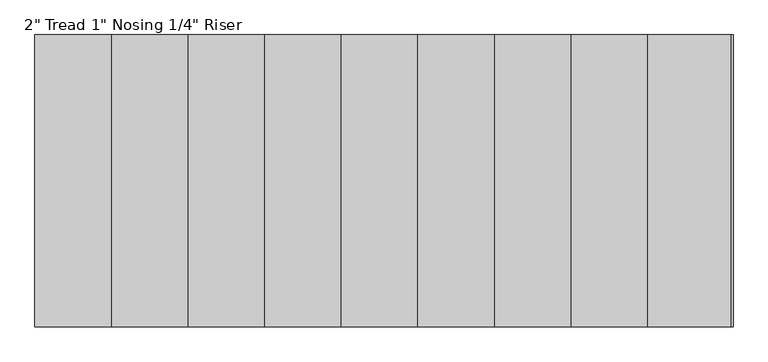
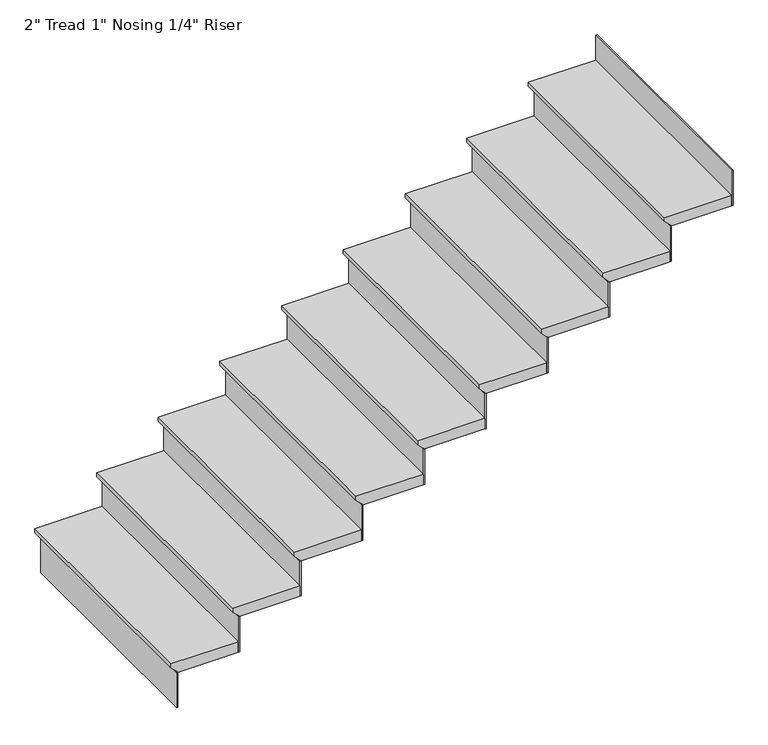
"""IFC4 building model written with IfcOpenShell, lengths in millimetres: stair flight geometry."""

from ifc_helpers import new_model, si_unit, frame, origin, place, context, project, spatial, polyline, outline, extrude, source, transform, mapped, element, save


def stair_flight_e984555f(model_context):
    return source(origin(), model_context, "Body", "SweptSolid", [
        extrude(outline(polyline([(1524.0, -13071.6750862), (1524.0, -13376.4750862), (1504.95, -13376.4750862), (1479.55, -13351.0750862), (1473.2, -13351.0750862), (1473.2, -13071.6750862), (1524.0, -13071.6750862)])), frame((0.0, 7319.8620171, 0.0), z_axis=(0.0, 1.0, 0.0), x_axis=(0.0, 0.0, 1.0)), (0.0, 0.0, 1.0), 1066.8),
        extrude(outline(polyline([(-13344.7250862, 7319.8620171), (-13351.0750862, 7319.8620171), (-13351.0750862, 8386.6620171), (-13344.7250862, 8386.6620171), (-13344.7250862, 7319.8620171)])), frame((0.0, 0.0, 1303.8666667), z_axis=(0.0, 0.0, 1.0), x_axis=(1.0, 0.0, 0.0)), (0.0, 0.0, 1.0), 169.3333333),
        extrude(outline(polyline([(-10830.1250862, 7319.8620171), (-10836.4750862, 7319.8620171), (-10836.4750862, 8386.6620171), (-10830.1250862, 8386.6620171), (-10830.1250862, 7319.8620171)])), frame((0.0, 0.0, 2827.8666667), z_axis=(0.0, 0.0, 1.0), x_axis=(1.0, 0.0, 0.0)), (0.0, 0.0, 1.0), 169.3333333),
        extrude(outline(polyline([(-13065.3250862, 7319.8620171), (-13071.6750862, 7319.8620171), (-13071.6750862, 8386.6620171), (-13065.3250862, 8386.6620171), (-13065.3250862, 7319.8620171)])), frame((0.0, 0.0, 1473.2), z_axis=(0.0, 0.0, 1.0), x_axis=(1.0, 0.0, 0.0)), (0.0, 0.0, 1.0), 169.3333333),
        extrude(outline(polyline([(1693.3333333, -12792.2750862), (1693.3333333, -13097.0750862), (1674.2833333, -13097.0750862), (1648.8833333, -13071.6750862), (1642.5333333, -13071.6750862), (1642.5333333, -12792.2750862), (1693.3333333, -12792.2750862)])), frame((0.0, 7319.8620171, 0.0), z_axis=(0.0, 1.0, 0.0), x_axis=(0.0, 0.0, 1.0)), (0.0, 0.0, 1.0), 1066.8),
        extrude(outline(polyline([(-12785.9250862, 7319.8620171), (-12792.2750862, 7319.8620171), (-12792.2750862, 8386.6620171), (-12785.9250862, 8386.6620171), (-12785.9250862, 7319.8620171)])), frame((0.0, 0.0, 1642.5333333), z_axis=(0.0, 0.0, 1.0), x_axis=(1.0, 0.0, 0.0)), (0.0, 0.0, 1.0), 169.3333333),
        extrude(outline(polyline([(1862.6666667, -12512.8750862), (1862.6666667, -12817.6750862), (1843.6166667, -12817.6750862), (1818.2166667, -12792.2750862), (1811.8666667, -12792.2750862), (1811.8666667, -12512.8750862), (1862.6666667, -12512.8750862)])), frame((0.0, 7319.8620171, 0.0), z_axis=(0.0, 1.0, 0.0), x_axis=(0.0, 0.0, 1.0)), (0.0, 0.0, 1.0), 1066.8),
        extrude(outline(polyline([(-12506.5250862, 7319.8620171), (-12512.8750862, 7319.8620171), (-12512.8750862, 8386.6620171), (-12506.5250862, 8386.6620171), (-12506.5250862, 7319.8620171)])), frame((0.0, 0.0, 1811.8666667), z_axis=(0.0, 0.0, 1.0), x_axis=(1.0, 0.0, 0.0)), (0.0, 0.0, 1.0), 169.3333333),
        extrude(outline(polyline([(2032.0, -12233.4750862), (2032.0, -12538.2750862), (2012.95, -12538.2750862), (1987.55, -12512.8750862), (1981.2, -12512.8750862), (1981.2, -12233.4750862), (2032.0, -12233.4750862)])), frame((0.0, 7319.8620171, 0.0), z_axis=(0.0, 1.0, 0.0), x_axis=(0.0, 0.0, 1.0)), (0.0, 0.0, 1.0), 1066.8),
        extrude(outline(polyline([(-12227.1250862, 7319.8620171), (-12233.4750862, 7319.8620171), (-12233.4750862, 8386.6620171), (-12227.1250862, 8386.6620171), (-12227.1250862, 7319.8620171)])), frame((0.0, 0.0, 1981.2), z_axis=(0.0, 0.0, 1.0), x_axis=(1.0, 0.0, 0.0)), (0.0, 0.0, 1.0), 169.3333333),
        extrude(outline(polyline([(2201.3333333, -11954.0750862), (2201.3333333, -12258.8750862), (2182.2833333, -12258.8750862), (2156.8833333, -12233.4750862), (2150.5333333, -12233.4750862), (2150.5333333, -11954.0750862), (2201.3333333, -11954.0750862)])), frame((0.0, 7319.8620171, 0.0), z_axis=(0.0, 1.0, 0.0), x_axis=(0.0, 0.0, 1.0)), (0.0, 0.0, 1.0), 1066.8),
        extrude(outline(polyline([(-11947.7250862, 7319.8620171), (-11954.0750862, 7319.8620171), (-11954.0750862, 8386.6620171), (-11947.7250862, 8386.6620171), (-11947.7250862, 7319.8620171)])), frame((0.0, 0.0, 2150.5333333), z_axis=(0.0, 0.0, 1.0), x_axis=(1.0, 0.0, 0.0)), (0.0, 0.0, 1.0), 169.3333333),
        extrude(outline(polyline([(2370.6666667, -11674.6750862), (2370.6666667, -11979.4750862), (2351.6166667, -11979.4750862), (2326.2166667, -11954.0750862), (2319.8666667, -11954.0750862), (2319.8666667, -11674.6750862), (2370.6666667, -11674.6750862)])), frame((0.0, 7319.8620171, 0.0), z_axis=(0.0, 1.0, 0.0), x_axis=(0.0, 0.0, 1.0)), (0.0, 0.0, 1.0), 1066.8),
        extrude(outline(polyline([(-11668.3250862, 7319.8620171), (-11674.6750862, 7319.8620171), (-11674.6750862, 8386.6620171), (-11668.3250862, 8386.6620171), (-11668.3250862, 7319.8620171)])), frame((0.0, 0.0, 2319.8666667), z_axis=(0.0, 0.0, 1.0), x_axis=(1.0, 0.0, 0.0)), (0.0, 0.0, 1.0), 169.3333333),
        extrude(outline(polyline([(2540.0, -11395.2750862), (2540.0, -11700.0750862), (2520.95, -11700.0750862), (2495.55, -11674.6750862), (2489.2, -11674.6750862), (2489.2, -11395.2750862), (2540.0, -11395.2750862)])), frame((0.0, 7319.8620171, 0.0), z_axis=(0.0, 1.0, 0.0), x_axis=(0.0, 0.0, 1.0)), (0.0, 0.0, 1.0), 1066.8),
        extrude(outline(polyline([(-11388.9250862, 7319.8620171), (-11395.2750862, 7319.8620171), (-11395.2750862, 8386.6620171), (-11388.9250862, 8386.6620171), (-11388.9250862, 7319.8620171)])), frame((0.0, 0.0, 2489.2), z_axis=(0.0, 0.0, 1.0), x_axis=(1.0, 0.0, 0.0)), (0.0, 0.0, 1.0), 169.3333333),
        extrude(outline(polyline([(2709.3333333, -11115.8750862), (2709.3333333, -11420.6750862), (2690.2833333, -11420.6750862), (2664.8833333, -11395.2750862), (2658.5333333, -11395.2750862), (2658.5333333, -11115.8750862), (2709.3333333, -11115.8750862)])), frame((0.0, 7319.8620171, 0.0), z_axis=(0.0, 1.0, 0.0), x_axis=(0.0, 0.0, 1.0)), (0.0, 0.0, 1.0), 1066.8),
        extrude(outline(polyline([(-11109.5250862, 7319.8620171), (-11115.8750862, 7319.8620171), (-11115.8750862, 8386.6620171), (-11109.5250862, 8386.6620171), (-11109.5250862, 7319.8620171)])), frame((0.0, 0.0, 2658.5333333), z_axis=(0.0, 0.0, 1.0), x_axis=(1.0, 0.0, 0.0)), (0.0, 0.0, 1.0), 169.3333333),
        extrude(outline(polyline([(2878.6666667, -10836.4750862), (2878.6666667, -11141.2750862), (2859.6166667, -11141.2750862), (2834.2166667, -11115.8750862), (2827.8666667, -11115.8750862), (2827.8666667, -10836.4750862), (2878.6666667, -10836.4750862)])), frame((0.0, 7319.8620171, 0.0), z_axis=(0.0, 1.0, 0.0), x_axis=(0.0, 0.0, 1.0)), (0.0, 0.0, 1.0), 1066.8),
    ])


if __name__ == "__main__":
    model = new_model("IFC4")
    model_context = context("Model", 3, world=origin())
    ifc_project = project(units=[si_unit("LENGTHUNIT", "METRE", prefix="MILLI")], contexts=[model_context])
    site = spatial("IfcSite", under=ifc_project)
    building = spatial("IfcBuilding", under=site)
    placement = place(None, origin())
    stair_flight_shape = stair_flight_e984555f(model_context)
    element("IfcStairFlight", 1, ObjectType="2\" Tread 1\" Nosing 1/4\" Riser", at=placement, inside=building, context=model_context, shape_type="MappedRepresentation", body=[
        mapped(stair_flight_shape, transform((0.0, 0.0, 0.0), x_axis=(1.0, 0.0, 0.0), y_axis=(0.0, 1.0, 0.0), z_axis=(0.0, 0.0, 1.0))),
    ])
    save(model, "model.ifc")
